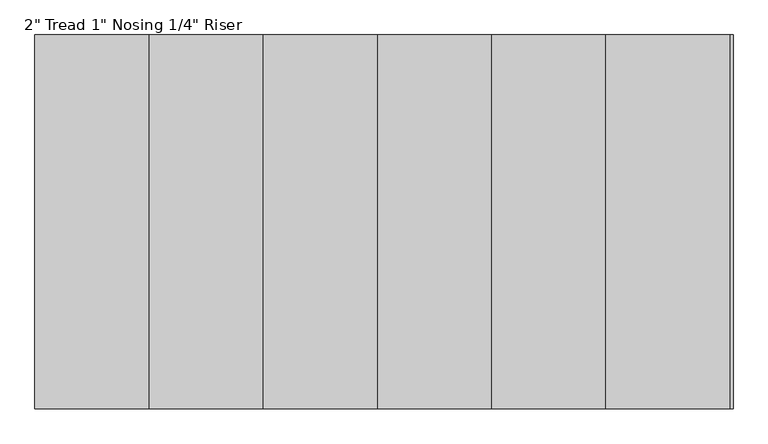
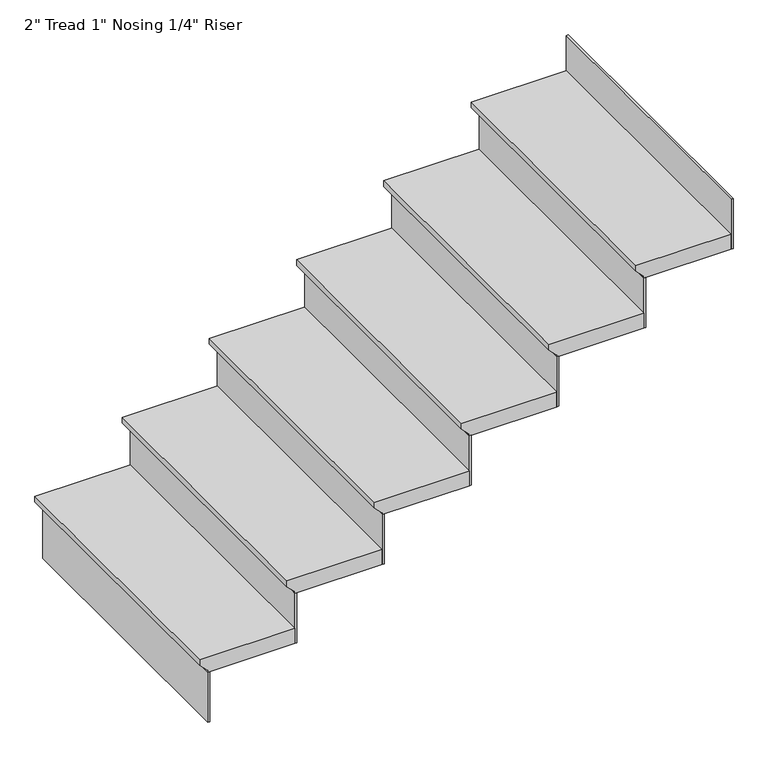
"""IFC4 building model written with IfcOpenShell, lengths in millimetres: stair flight geometry."""

from ifc_helpers import new_model, si_unit, frame, origin, place, context, project, spatial, polyline, outline, extrude, source, transform, mapped, element, save


def stair_flight_848efa21(model_context):
    return source(origin(), model_context, "Body", "SweptSolid", [
        extrude(outline(polyline([(8737.6, -8480.0517085), (8737.6, -8784.8517085), (8718.55, -8784.8517085), (8693.15, -8759.4517085), (8686.8, -8759.4517085), (8686.8, -8480.0517085), (8737.6, -8480.0517085)])), frame((0.0, 792.0165128, 0.0), z_axis=(0.0, 1.0, 0.0), x_axis=(0.0, 0.0, 1.0)), (0.0, 0.0, 1.0), 914.4),
        extrude(outline(polyline([(-8753.1017085, 792.0165128), (-8759.4517085, 792.0165128), (-8759.4517085, 1706.4165128), (-8753.1017085, 1706.4165128), (-8753.1017085, 792.0165128)])), frame((0.0, 0.0, 8517.4666667), z_axis=(0.0, 0.0, 1.0), x_axis=(1.0, 0.0, 0.0)), (0.0, 0.0, 1.0), 169.3333333),
        extrude(outline(polyline([(-8473.7017085, 792.0165128), (-8480.0517085, 792.0165128), (-8480.0517085, 1706.4165128), (-8473.7017085, 1706.4165128), (-8473.7017085, 792.0165128)])), frame((0.0, 0.0, 8686.8), z_axis=(0.0, 0.0, 1.0), x_axis=(1.0, 0.0, 0.0)), (0.0, 0.0, 1.0), 169.3333333),
        extrude(outline(polyline([(8906.9333333, -8200.6517085), (8906.9333333, -8505.4517085), (8887.8833333, -8505.4517085), (8862.4833333, -8480.0517085), (8856.1333333, -8480.0517085), (8856.1333333, -8200.6517085), (8906.9333333, -8200.6517085)])), frame((0.0, 792.0165128, 0.0), z_axis=(0.0, 1.0, 0.0), x_axis=(0.0, 0.0, 1.0)), (0.0, 0.0, 1.0), 914.4),
        extrude(outline(polyline([(-8194.3017085, 792.0165128), (-8200.6517085, 792.0165128), (-8200.6517085, 1706.4165128), (-8194.3017085, 1706.4165128), (-8194.3017085, 792.0165128)])), frame((0.0, 0.0, 8856.1333333), z_axis=(0.0, 0.0, 1.0), x_axis=(1.0, 0.0, 0.0)), (0.0, 0.0, 1.0), 169.3333333),
        extrude(outline(polyline([(9076.2666667, -7921.2517085), (9076.2666667, -8226.0517085), (9057.2166667, -8226.0517085), (9031.8166667, -8200.6517085), (9025.4666667, -8200.6517085), (9025.4666667, -7921.2517085), (9076.2666667, -7921.2517085)])), frame((0.0, 792.0165128, 0.0), z_axis=(0.0, 1.0, 0.0), x_axis=(0.0, 0.0, 1.0)), (0.0, 0.0, 1.0), 914.4),
        extrude(outline(polyline([(-7914.9017085, 792.0165128), (-7921.2517085, 792.0165128), (-7921.2517085, 1706.4165128), (-7914.9017085, 1706.4165128), (-7914.9017085, 792.0165128)])), frame((0.0, 0.0, 9025.4666667), z_axis=(0.0, 0.0, 1.0), x_axis=(1.0, 0.0, 0.0)), (0.0, 0.0, 1.0), 169.3333333),
        extrude(outline(polyline([(9245.6, -7641.8517085), (9245.6, -7946.6517085), (9226.55, -7946.6517085), (9201.15, -7921.2517085), (9194.8, -7921.2517085), (9194.8, -7641.8517085), (9245.6, -7641.8517085)])), frame((0.0, 792.0165128, 0.0), z_axis=(0.0, 1.0, 0.0), x_axis=(0.0, 0.0, 1.0)), (0.0, 0.0, 1.0), 914.4),
        extrude(outline(polyline([(-7635.5017085, 792.0165128), (-7641.8517085, 792.0165128), (-7641.8517085, 1706.4165128), (-7635.5017085, 1706.4165128), (-7635.5017085, 792.0165128)])), frame((0.0, 0.0, 9194.8), z_axis=(0.0, 0.0, 1.0), x_axis=(1.0, 0.0, 0.0)), (0.0, 0.0, 1.0), 169.3333333),
        extrude(outline(polyline([(9414.9333333, -7362.4517085), (9414.9333333, -7667.2517085), (9395.8833333, -7667.2517085), (9370.4833333, -7641.8517085), (9364.1333333, -7641.8517085), (9364.1333333, -7362.4517085), (9414.9333333, -7362.4517085)])), frame((0.0, 792.0165128, 0.0), z_axis=(0.0, 1.0, 0.0), x_axis=(0.0, 0.0, 1.0)), (0.0, 0.0, 1.0), 914.4),
        extrude(outline(polyline([(-7356.1017085, 792.0165128), (-7362.4517085, 792.0165128), (-7362.4517085, 1706.4165128), (-7356.1017085, 1706.4165128), (-7356.1017085, 792.0165128)])), frame((0.0, 0.0, 9364.1333333), z_axis=(0.0, 0.0, 1.0), x_axis=(1.0, 0.0, 0.0)), (0.0, 0.0, 1.0), 169.3333333),
        extrude(outline(polyline([(-7076.7017085, 792.0165128), (-7083.0517085, 792.0165128), (-7083.0517085, 1706.4165128), (-7076.7017085, 1706.4165128), (-7076.7017085, 792.0165128)])), frame((0.0, 0.0, 9533.4666667), z_axis=(0.0, 0.0, 1.0), x_axis=(1.0, 0.0, 0.0)), (0.0, 0.0, 1.0), 169.3333333),
        extrude(outline(polyline([(9584.2666667, -7083.0517085), (9584.2666667, -7387.8517085), (9565.2166667, -7387.8517085), (9539.8166667, -7362.4517085), (9533.4666667, -7362.4517085), (9533.4666667, -7083.0517085), (9584.2666667, -7083.0517085)])), frame((0.0, 792.0165128, 0.0), z_axis=(0.0, 1.0, 0.0), x_axis=(0.0, 0.0, 1.0)), (0.0, 0.0, 1.0), 914.4),
    ])


if __name__ == "__main__":
    model = new_model("IFC4")
    model_context = context("Model", 3, world=origin())
    ifc_project = project(units=[si_unit("LENGTHUNIT", "METRE", prefix="MILLI")], contexts=[model_context])
    site = spatial("IfcSite", under=ifc_project)
    building = spatial("IfcBuilding", under=site)
    placement = place(None, origin())
    stair_flight_shape = stair_flight_848efa21(model_context)
    element("IfcStairFlight", 1, ObjectType="2\" Tread 1\" Nosing 1/4\" Riser", at=placement, inside=building, context=model_context, shape_type="MappedRepresentation", body=[
        mapped(stair_flight_shape, transform((0.0, 0.0, 0.0), x_axis=(1.0, 0.0, 0.0), y_axis=(0.0, 1.0, 0.0), z_axis=(0.0, 0.0, 1.0))),
    ])
    save(model, "model.ifc")
